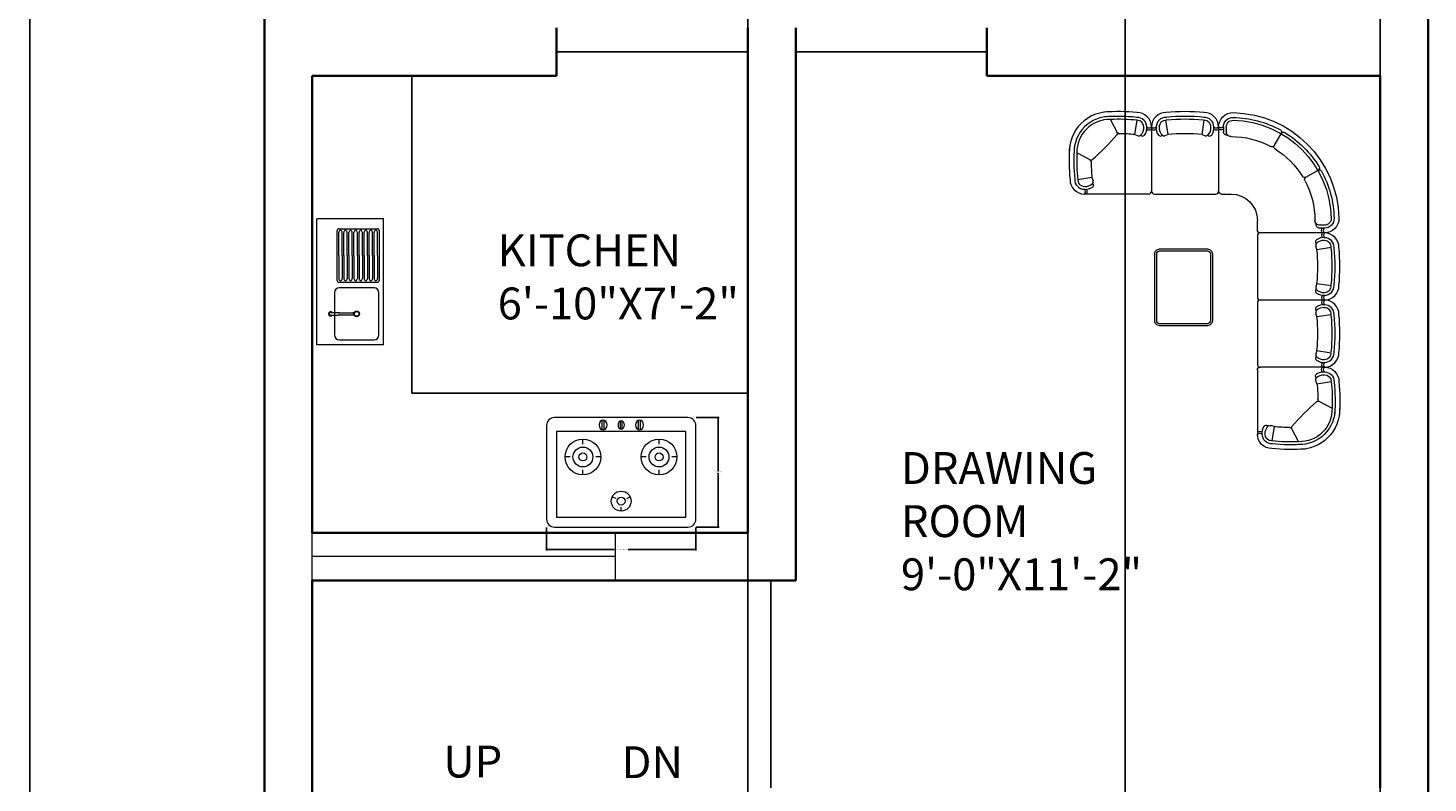
# Model space of a CAD drawing. Units: inches. Extents: x -16 to 587, y -783 to 64.
# Tile 9 of 14: x 279 to 543, y -534 to -392. Entities that reach past the tile are written whole.
import ezdxf

# ---------------------------------------------------------------- set-up
doc = ezdxf.new("R2010")
doc.units = ezdxf.units.IN
doc.header["$MEASUREMENT"] = 0
for name, color, linetype, lineweight in [('A-ANNO-DIMS', 2, 'Continuous', 18), ('A-ANNO-SYMB', 7, 'Continuous', 18), ('A-ANNO-TEXT', 7, 'Continuous', 25), ('A-AREA-IDEN', 7, 'Continuous', 18), ('A-DOOR', 3, 'Continuous', 25), ('A-EQPM', 8, 'Continuous', 18), ('A-FLOR-CASE', 7, 'Continuous', 25), ('A-FLOR-FIXT', 9, 'Continuous', 18), ('A-FURN', 8, 'Continuous', 18), ('A-GLAZ', 4, 'Continuous', 18), ('A-WALL', 7, 'Continuous', 35)]:
    doc.layers.add(name, color=color, linetype=linetype, lineweight=lineweight)
doc.styles.get("Standard").update_dxf_attribs({"font": 'arial.ttf'})
doc.dimstyles.get("Standard").update_dxf_attribs({"dimtxt": 0.18, "dimasz": 0.18, "dimexe": 0.18, "dimexo": 0.0625, "dimgap": 0.09, "dimtad": 0, "dimtih": 1, "dimtoh": 1, "dimdec": 0, "dimzin": 0, "dimdsep": 46, "dimlunit": 3, "dimtxsty": 'Standard', "dimcen": 0.09, "dimadec": 0, "dimazin": 0, "dimtfac": 1, "dimtdec": 0, "dimtofl": 0, "dimtmove": 0, "dimatfit": 3, "dimfxl": 1, "dimtolj": 1, "dimtzin": 0, "dimarcsym": 0})

# ---------------------------------------------------------------- blocks, each defined once
blk = doc.blocks.new('A$C707258B2')
at = {"color": 0}
for p, q in [((0.404, 0.342), (1.074, 0.342)), ((1.104, 0.312), (1.104, 0.212)), ((0.404, 0.292), (0.454, 0.292)), ((0.404, 0.262), (0.454, 0.262)), ((1.479, -0.063), (1.379, -0.063)), ((1.509, -0.763), (1.509, -0.093)), ((0.6, -0.238), (0.47, -0.313)), ((0.929, -0.567), (0.854, -0.697)), ((1.429, -0.763), (1.429, -0.713)), ((1.459, -0.763), (1.459, -0.712))]:
    blk.add_line(p, q, dxfattribs=at)
for centre, radius, start, end in [((0.404, 0.192), 0.15, 90, 181.1754), ((0.378, 0.317), 0.0362, 316.3972, 43.6028), ((0.368, 0.317), 0.0662, 337.8298, 22.1702), ((1.074, 0.312), 0.03, 360, 90), ((1.379, 0.212), 1.125, 181.1754, 268.8246), ((0.404, 0.192), 0.1, 90, 181.1754), ((1.379, 0.212), 1.075, 181.1754, 208.6357), ((0.404, 0.192), 0.07, 90, 181.1754), ((1.379, 0.212), 1.045, 181.1754, 268.8246), ((0.455, 0.256), 0.0357, 345.4262, 90.5555), ((0.454, 0.212), 0.05, 360, 90), ((1.379, 0.212), 0.875, 180, 208.4082), ((1.379, 0.212), 0.275, 180, 270), ((1.479, -0.093), 0.03, 360, 90), ((0.587, -0.216), 0.025, 300, 28.4082), ((0.612, -0.259), 0.025, 31.5918, 120), ((1.379, 0.212), 0.875, 211.5918, 238.4082), ((0.457, -0.291), 0.025, 208.6357, 300), ((0.482, -0.334), 0.025, 120, 211.3643), ((1.379, 0.212), 1.075, 211.3643, 238.6357), ((0.907, -0.555), 0.025, 330, 58.4082), ((0.951, -0.58), 0.025, 61.5918, 150), ((1.379, 0.212), 0.875, 241.5918, 270), ((0.832, -0.685), 0.025, 238.6357, 330), ((0.876, -0.71), 0.025, 150, 241.3643), ((1.379, -0.713), 0.05, 360, 90), ((1.425, -0.709), 0.0336, 354.6301, 109.3883), ((1.379, 0.212), 1.075, 241.3643, 268.8246), ((1.359, -0.763), 0.15, 268.8246, 360), ((1.359, -0.763), 0.1, 268.8246, 360), ((1.359, -0.763), 0.07, 268.8246, 360), ((1.484, -0.799), 0.0662, 67.8298, 112.1702), ((1.484, -0.789), 0.0362, 46.3972, 133.6028)]:
    blk.add_arc(centre, radius, start, end, dxfattribs=at)
blk = doc.blocks.new('A$C1352')
at = {"color": 0}
for points in [[(0.003, 0.053), (0.003, 0.553, -0.414214), (0.053, 0.603), (0.753, 0.603, -0.414214), (0.803, 0.553), (0.803, 0.053, -0.414214), (0.753, 0.003), (0.053, 0.003, -0.414214)], [(0.023, 0.053), (0.023, 0.553, -0.414214), (0.053, 0.583), (0.753, 0.583, -0.414214), (0.783, 0.553), (0.783, 0.053, -0.414214), (0.753, 0.023), (0.053, 0.023, -0.414214)]]:
    blk.add_lwpolyline(points, format="xyb", close=True, dxfattribs=at)
blk = doc.blocks.new('part 01')
at = {"color": 0}
for p, q in [((-670, 700), (0, 700)), ((30, 30), (30, 670)), ((-591, 527), (-740, 550)), ((-591, 527), (-579, 561)), ((-591, 173), (-740, 150)), ((-591, 173), (-579, 139)), ((-670, 0), (0, 0))]:
    blk.add_line(p, q, dxfattribs=at)
for centre, radius, start, end in [((-670, 550), 150, 90, 181.1754), ((-670, 550), 100, 90, 181.1754), ((-670, 550), 70, 90, 181.1754), ((-660, 518), 133, 56.0897, 95.6132), ((-696, 675), 36.2, 316.3972, 43.6028), ((-660, 518), 103, 42.0066, 95.6132), ((-706, 675), 66.2, 337.8298, 22.1702), ((-600, 607), 25, 332.9608, 56.0897), ((-625, 620), 53.2, 321.0017, 332.9608), ((-602, 570), 25, 340, 42.0066), ((0, 670), 30, 0, 90), ((1178, 350), 2008, 174.2835, 185.7165), ((1178, 350), 1958, 174.2835, 185.7165), ((1178, 350), 1928, 174.2835, 185.7165), ((1178, 350), 1778, 174.2835, 185.7165), ((-670, 150), 150, 178.8246, 270), ((-670, 150), 100, 178.8246, 270), ((-670, 150), 70, 178.8246, 270), ((-660, 182), 133, 264.3868, 303.9103), ((-660, 182), 103, 264.3868, 317.9934), ((-696, 25), 36.2, 316.3972, 43.6028), ((-706, 25), 66.2, 337.8298, 22.1702), ((-600, 93), 25, 303.9103, 27.0392), ((-602, 130), 25, 317.9934, 20), ((-625, 80), 53.2, 27.0392, 38.9983), ((0, 30), 30, 270, 0)]:
    blk.add_arc(centre, radius, start, end, dxfattribs=at)
blk = doc.blocks.new('part02')
at = {"color": 0}
for p, q in [((0, -670), (0, 0)), ((30, 30), (700, 30)), ((621, -143), (609, -109)), ((621, -143), (770, -120)), ((640, -326), (778, -399)), ((173, -591), (139, -579)), ((173, -591), (150, -740)), ((356, -610), (429, -748))]:
    blk.add_line(p, q, dxfattribs=at)
for centre, radius, start, end in [((30, 0), 30, 90, 180), ((726, 5), 56.2, 153.6122, 206.6666), ((726, 5), 36.2, 136.3972, 223.6028), ((700, -120), 150, 0, 90), ((630, -63), 25, 123.9103, 207.0392), ((655, -50), 53.2, 207.0392, 218.9983), ((632, -100), 25, 137.9934, 200), ((690, -152), 103, 84.3868, 137.9934), ((689, -151), 132, 85.4378, 123.9887), ((-1148, -320), 1778, 0.3836, 5.7165), ((700, -121), 101, 357.5006, 89.858), ((700, -120), 70, 0, 90), ((-1228, -320), 2008, 357.7349, 5.7032), ((-1148, -320), 1958, 355.8657, 5.7165), ((-1148, -320), 2008, 355.818, 5.7165), ((2220, -2190), 2454, 130.6961, 139.3039), ((439, -409), 419, 268.2181, 1.7819), ((439, -409), 369, 268.2181, 1.7819), ((439, -409), 339, 268.2181, 1.7819), ((632, -344), 20, 62, 130.6961), ((650, -308), 20, 180.3836, 242), ((93, -600), 25, 62.9608, 146.0897), ((182, -660), 103, 132.0066, 185.6132), ((80, -625), 53.2, 51.0017, 62.9608), ((130, -602), 25, 70, 132.0066), ((25, -696), 56.2, 63.3334, 116.3878), ((25, -696), 36.2, 46.3972, 133.6028), ((150, -670), 150, 180, 271.1754), ((182, -660), 133, 146.0897, 185.6132), ((150, -670), 100, 180, 271.1754), ((150, -670), 70, 180, 270), ((350, 1178), 1778, 264.2835, 269.6164), ((338, -620), 20, 28, 89.6164), ((374, -602), 20, 139.3039, 208), ((350, 1258), 2008, 264.2968, 272.2651), ((350, 1178), 2008, 264.2835, 274.182), ((350, 1178), 1958, 264.2835, 274.1343)]:
    blk.add_arc(centre, radius, start, end, dxfattribs=at)
blk = doc.blocks.new('KITCHEN-SINK')
for p, q in [((12.53, 23.71), (0, 23.71)), ((0, 0), (0, 23.71)), ((3.76, 21.39), (3.76, 12.19)), ((4.1, 16.79), (4.1, 21.13)), ((4.19, 21.83), (11.32, 21.83)), ((4.75, 16.79), (4.75, 21.13)), ((5.05, 16.79), (5.05, 21.13)), ((5.7, 16.79), (5.7, 21.13)), ((6, 16.79), (6, 21.13)), ((6.65, 16.79), (6.65, 21.13)), ((6.96, 16.79), (6.96, 21.13)), ((7.6, 16.79), (7.6, 21.13)), ((7.91, 16.79), (7.91, 21.13)), ((8.56, 16.79), (8.56, 21.13)), ((8.86, 16.79), (8.86, 21.13)), ((9.51, 16.79), (9.51, 21.13)), ((9.81, 16.79), (9.81, 21.13)), ((10.46, 16.79), (10.46, 21.13)), ((10.76, 16.79), (10.76, 21.13)), ((11.41, 16.79), (11.41, 21.13)), ((11.75, 12.19), (11.75, 21.39)), ((12.53, 0), (12.53, 23.71)), ((4.1, 16.79), (4.1, 12.45)), ((4.75, 16.79), (4.75, 12.45)), ((5.05, 16.79), (5.05, 12.45)), ((5.7, 16.79), (5.7, 12.45)), ((6, 16.79), (6, 12.45)), ((6.65, 16.79), (6.65, 12.45)), ((6.96, 16.79), (6.96, 12.45)), ((7.6, 16.79), (7.6, 12.45)), ((7.91, 16.79), (7.91, 12.45)), ((8.56, 16.79), (8.56, 12.45)), ((8.86, 16.79), (8.86, 12.45)), ((9.51, 16.79), (9.51, 12.45)), ((9.81, 16.79), (9.81, 12.45)), ((10.46, 16.79), (10.46, 12.45)), ((10.76, 16.79), (10.76, 12.45)), ((11.41, 16.79), (11.41, 12.45)), ((4.19, 11.76), (11.32, 11.76)), ((10.73, 10.7), (4.21, 10.7)), ((3.28, 9.77), (3.28, 6.06)), ((11.66, 1.84), (11.66, 9.77)), ((3.28, 5.95), (3.28, 1.84)), ((4.21, 0.91), (10.73, 0.91)), ((12.53, 0), (0, 0))]:
    blk.add_line(p, q)
for points in [[(2.55, 6.06), (3.98, 6.06)], [(2.55, 5.54), (3.98, 5.54)], [(4.14, 6), (6.76, 6)], [(4.14, 5.61), (6.76, 5.61)]]:
    blk.add_lwpolyline(points)
for radius in [0.54, 0.432]:
    blk.add_circle((7.47, 5.8), radius)
for centre, radius, start, end in [((4.19, 21.39), 0.432, 90, 180), ((4.53, 21.13), 0.432, 104.4903, 180), ((4.32, 21.13), 0.432, 0, 75.5097), ((5.48, 21.13), 0.432, 104.4903, 180), ((5.27, 21.13), 0.432, 0, 75.5097), ((6.44, 21.13), 0.432, 104.4903, 180), ((6.22, 21.13), 0.432, 0, 75.5097), ((7.39, 21.13), 0.432, 104.4903, 180), ((7.17, 21.13), 0.432, 0, 75.5097), ((8.34, 21.13), 0.432, 104.4903, 180), ((8.12, 21.13), 0.432, 0, 75.5097), ((9.29, 21.13), 0.432, 104.4903, 180), ((9.07, 21.13), 0.432, 0, 75.5097), ((10.24, 21.13), 0.432, 104.4903, 180), ((10.03, 21.13), 0.432, 0, 75.5097), ((11.19, 21.13), 0.432, 104.4903, 180), ((10.98, 21.13), 0.432, 0, 75.5097), ((11.32, 21.39), 0.432, 0, 90), ((4.21, 9.77), 0.933, 90, 180), ((4.19, 12.19), 0.432, 180, 270), ((4.53, 12.45), 0.432, 180, 255.5097), ((4.32, 12.45), 0.432, 284.4903, 0), ((5.48, 12.45), 0.432, 180, 255.5097), ((5.27, 12.45), 0.432, 284.4903, 0), ((6.44, 12.45), 0.432, 180, 255.5097), ((6.22, 12.45), 0.432, 284.4903, 0), ((7.39, 12.45), 0.432, 180, 255.5097), ((7.17, 12.45), 0.432, 284.4903, 0), ((8.34, 12.45), 0.432, 180, 255.5097), ((8.12, 12.45), 0.432, 284.4903, 0), ((9.29, 12.45), 0.432, 180, 255.5097), ((9.07, 12.45), 0.432, 284.4903, 0), ((10.24, 12.45), 0.432, 180, 255.5097), ((10.03, 12.45), 0.432, 284.4903, 0), ((10.73, 9.77), 0.933, 0, 90), ((11.19, 12.45), 0.432, 180, 255.5097), ((10.98, 12.45), 0.432, 284.4903, 0), ((11.32, 12.19), 0.432, 270, 0), ((2.55, 5.8), 0.388, 41.9018, 318.0982), ((2.55, 5.8), 0.259, 90, 270), ((3.97, 5.8), 0.259, 272.2198, 87.7802), ((6.78, 5.8), 0.195, 264.9463, 95.0537), ((4.21, 1.84), 0.933, 180, 270), ((10.73, 1.84), 0.933, 270, 0)]:
    blk.add_arc(centre, radius, start, end)
blk = doc.blocks.new('COOKTOP-THREE-BURNER')
for p, q in [((0, 19.11), (0, 1.5)), ((26.61, 20.61), (1.5, 20.61)), ((10.46, 18.28), (10.46, 20.15)), ((10.83, 18.28), (10.83, 20.15)), ((13.92, 18.45), (13.92, 19.97)), ((14.22, 18.45), (14.22, 19.97)), ((17.32, 18.28), (17.32, 20.15)), ((17.7, 18.28), (17.7, 20.15)), ((28.11, 1.5), (28.11, 19.11)), ((26.23, 17.99), (1.87, 17.99)), ((1.87, 17.99), (1.87, 1.87)), ((6.85, 15.63), (6.85, 16.56)), ((21.18, 15.63), (21.18, 16.56)), ((26.23, 1.87), (26.23, 17.99)), ((4.42, 13.19), (3.48, 13.19)), ((10.23, 13.19), (9.29, 13.19)), ((18.74, 13.19), (17.8, 13.19)), ((24.55, 13.19), (23.61, 13.19)), ((6.85, 9.82), (6.85, 10.76)), ((21.18, 9.82), (21.18, 10.76)), ((12.37, 5.69), (13.06, 5.41)), ((15.74, 5.69), (15.08, 5.34)), ((14.05, 3), (14.05, 3.75)), ((1.5, 0), (26.61, 0)), ((1.87, 1.87), (26.23, 1.87))]:
    blk.add_line(p, q)
for centre, radius in [((6.85, 13.19), 3.37), ((21.18, 13.19), 3.37), ((6.85, 13.19), 1.87), ((6.85, 13.19), 0.75), ((21.18, 13.19), 1.87), ((21.18, 13.19), 0.75), ((14.05, 4.88), 1.87), ((14.05, 4.88), 0.75)]:
    blk.add_circle(centre, radius)
for centre, start, end in [((1.5, 19.11), 90, 180), ((26.61, 19.11), 0, 90), ((1.5, 1.5), 180, 270), ((26.61, 1.5), 270, 0)]:
    blk.add_arc(centre, 1.5, start, end)
at = {"extrusion": (0, 0, -1)}
for centre, major_axis in [((10.65, 19.21), (0, 0.937)), ((14.07, 19.21), (0, 0.759)), ((17.51, 19.21), (0, 0.937))]:
    blk.add_ellipse(centre, major_axis=major_axis, ratio=0.802399, dxfattribs=at)
blk = doc.blocks.new('*D40')
at = {"layer": 'A-ANNO-DIMS', "color": 0, "lineweight": -2, "transparency": 16777216}
for p, q in [((376.89, -485.54), (376.89, -489.87)), ((405, -485.54), (405, -489.87)), ((377.07, -489.69), (389.64, -489.69)), ((404.82, -489.69), (392.24, -489.69))]:
    blk.add_line(p, q, dxfattribs=at)
at = {"layer": 'A-ANNO-DIMS', "color": 0, "transparency": 16777216}
for points in [[(377.07, -489.66), (377.07, -489.72), (376.89, -489.69)], [(404.82, -489.66), (404.82, -489.72), (405, -489.69)]]:
    blk.add_solid(points, dxfattribs=at)
at = {"layer": 'Defpoints', "color": 0, "transparency": 16777216}
for p in [(376.89, -485.48), (405, -485.48), (405, -489.69)]:
    blk.add_point(p, dxfattribs=at)
at = {"layer": 'A-ANNO-DIMS', "color": 0, "transparency": 16777216, "insert": (390.94, -489.69), "char_height": 0.18, "attachment_point": 5}
blk.add_mtext('\\A1;COOKTOP 2\'-4" TYP.', dxfattribs=at)
blk = doc.blocks.new('*D41')
at = {"layer": 'A-ANNO-DIMS', "color": 0, "lineweight": -2, "transparency": 16777216}
for p, q in [((405.06, -464.86), (409.39, -464.86)), ((409.21, -465.04), (409.21, -474.99)), ((409.21, -485.3), (409.21, -475.35)), ((405.06, -485.48), (409.39, -485.48))]:
    blk.add_line(p, q, dxfattribs=at)
at = {"layer": 'A-ANNO-DIMS', "color": 0, "transparency": 16777216}
for points in [[(409.18, -465.04), (409.24, -465.04), (409.21, -464.86)], [(409.18, -485.3), (409.24, -485.3), (409.21, -485.48)]]:
    blk.add_solid(points, dxfattribs=at)
at = {"layer": 'Defpoints', "color": 0, "transparency": 16777216}
for p in [(405, -464.86), (409.21, -464.86), (405, -485.48)]:
    blk.add_point(p, dxfattribs=at)
at = {"layer": 'A-ANNO-DIMS', "color": 0, "transparency": 16777216, "insert": (409.21, -475.17), "char_height": 0.18, "attachment_point": 5}
blk.add_mtext('\\A1;1\'-8 1/2" TYP.', dxfattribs=at)
blk = doc.blocks.new('*D53')
at = {"layer": 'A-ANNO-DIMS', "color": 0, "lineweight": -2, "transparency": 16777216}
for p, q in [((323.73, 19.45), (279.46, 19.45)), ((279.64, 19.27), (279.64, -358.87)), ((279.64, -737.37), (279.64, -359.24)), ((323.73, -737.55), (279.46, -737.55))]:
    blk.add_line(p, q, dxfattribs=at)
at = {"layer": 'A-ANNO-DIMS', "color": 0, "transparency": 16777216}
for points in [[(279.61, 19.27), (279.67, 19.27), (279.64, 19.45)], [(279.61, -737.37), (279.67, -737.37), (279.64, -737.55)]]:
    blk.add_solid(points, dxfattribs=at)
at = {"layer": 'Defpoints', "color": 0, "transparency": 16777216}
for p in [(323.79, 19.45), (279.64, -737.55), (323.79, -737.55)]:
    blk.add_point(p, dxfattribs=at)
at = {"layer": 'A-ANNO-DIMS', "color": 0, "transparency": 16777216, "insert": (279.64, -359.05), "char_height": 0.18, "attachment_point": 5}
blk.add_mtext('\\A1;63\'-1"', dxfattribs=at)
blk = doc.blocks.new('*D55')
at = {"layer": 'A-ANNO-DIMS', "color": 0, "lineweight": -2, "transparency": 16777216}
for p, q in [((485.79, -75.62), (485.79, -781.88)), ((533.79, -75.62), (533.79, -781.88)), ((485.97, -781.7), (509.46, -781.7)), ((533.61, -781.7), (510.12, -781.7))]:
    blk.add_line(p, q, dxfattribs=at)
at = {"layer": 'A-ANNO-DIMS', "color": 0, "transparency": 16777216}
for points in [[(485.97, -781.67), (485.97, -781.73), (485.79, -781.7)], [(533.61, -781.67), (533.61, -781.73), (533.79, -781.7)]]:
    blk.add_solid(points, dxfattribs=at)
at = {"layer": 'Defpoints', "color": 0, "transparency": 16777216}
for p in [(485.79, -75.55), (533.79, -75.55), (533.79, -781.7)]:
    blk.add_point(p, dxfattribs=at)
at = {"layer": 'A-ANNO-DIMS', "color": 0, "transparency": 16777216, "insert": (509.79, -781.7), "char_height": 0.18, "attachment_point": 5}
blk.add_mtext('\\A1;4\'-0"', dxfattribs=at)
blk = doc.blocks.new('*D59')
at = {"layer": 'A-ANNO-DIMS', "color": 0, "lineweight": -2, "transparency": 16777216}
for p, q in [((414.79, -712.99), (414.79, 63.78)), ((414.97, 63.6), (478.4, 63.6)), ((542.61, 63.6), (479.18, 63.6)), ((542.79, -712.99), (542.79, 63.78))]:
    blk.add_line(p, q, dxfattribs=at)
at = {"layer": 'A-ANNO-DIMS', "color": 0, "transparency": 16777216}
for points in [[(414.97, 63.63), (414.97, 63.57), (414.79, 63.6)], [(542.61, 63.63), (542.61, 63.57), (542.79, 63.6)]]:
    blk.add_solid(points, dxfattribs=at)
at = {"layer": 'Defpoints', "color": 0, "transparency": 16777216}
for p in [(542.79, 63.6), (414.79, -713.05), (542.79, -713.05)]:
    blk.add_point(p, dxfattribs=at)
at = {"layer": 'A-ANNO-DIMS', "color": 0, "transparency": 16777216, "insert": (478.79, 63.6), "char_height": 0.18, "attachment_point": 5}
blk.add_mtext('\\A1;10\'-8"', dxfattribs=at)

msp = doc.modelspace()

# ---------------------------------------------------------------- linework, layer by layer
at = {"layer": 'A-ANNO-SYMB'}
msp.add_line((359.58, -529.79), (359.58, -529.79), dxfattribs=at)
at = {"layer": 'A-DOOR'}
for p, q in [((378.79, -396.05), (414.79, -396.05)), ((423.79, -396.05), (459.79, -396.05)), ((419.12, -534.55), (419.12, -495.55))]:
    msp.add_line(p, q, dxfattribs=at)
at = {"layer": 'A-FLOR-CASE'}
for p, q in [((351.52, -400.55), (351.52, -460.28)), ((351.52, -460.28), (414.79, -460.28))]:
    msp.add_line(p, q, dxfattribs=at)
at = {"layer": 'A-GLAZ'}
for p, q in [((332.79, -495.55), (332.79, -486.55)), ((332.79, -486.55), (389.81, -486.55)), ((389.81, -486.55), (389.81, -495.55)), ((389.81, -491.05), (332.79, -491.05)), ((389.81, -495.55), (332.79, -495.55))]:
    msp.add_line(p, q, dxfattribs=at)
at = {"layer": 'A-WALL'}
for p, q in [((323.79, 19.45), (323.79, -737.55)), ((542.79, 19.45), (542.79, -737.55)), ((378.79, -391.55), (378.79, -400.55)), ((414.79, -391.55), (414.79, -486.55)), ((423.79, -391.55), (423.79, -495.55)), ((459.79, -391.55), (459.79, -400.55)), ((332.79, -400.55), (378.79, -400.55)), ((332.79, -400.55), (332.79, -486.55)), ((459.79, -400.55), (476.79, -400.55)), ((476.79, -400.55), (533.79, -400.55)), ((533.79, -400.55), (533.79, -486.55)), ((332.79, -486.55), (414.79, -486.55)), ((533.79, -486.55), (533.79, -495.55)), ((332.79, -495.55), (423.79, -495.55)), ((332.79, -495.55), (332.79, -663.55)), ((533.79, -495.55), (533.79, -534.55))]:
    msp.add_line(p, q, dxfattribs=at)

# ---------------------------------------------------------------- block references
at = {"layer": 'A-EQPM'}
msp.add_blockref('COOKTOP-THREE-BURNER', (376.89, -485.48), dxfattribs=at)
at = {"layer": 'A-FLOR-FIXT'}
msp.add_blockref('KITCHEN-SINK', (333.69, -451.16), dxfattribs=at)
at = {"layer": 'A-FURN', "ltscale": 0.03}
for name, p, xscale, yscale, zscale, rotation in [('part02', (490.75, -422.27), 0.0180440482994306, 0.0180440482994306, 0.0180440482994306, 180), ('part 01', (490.75, -422.27), 0.0180440482994306, 0.0180440482994306, 0.0180440482994306, 270), ('A$C707258B2', (509.55, -402.89), -18.04404829943058, 18.04404829943058, 18.04404829943058, 89.9999999999967), ('part 01', (511.23, -430.12), 0.0180440482994306, 0.0180440482994306, 0.0180440482994306, 180), ('A$C1352', (491.32, -433.09), 18.04404829943058, 18.04404829943058, 18.04404829943058, 270), ('part 01', (511.23, -442.75), 0.0180440482994306, 0.0180440482994306, 0.0180440482994306, 180), ('part02', (511.23, -455.38), -0.0180440482994306, 0.0180440482994306, 0.0180440482994306, 89.9999999999967)]:
    msp.add_blockref(name, p, dxfattribs=dict(at, xscale=xscale, yscale=yscale, zscale=zscale, rotation=rotation))

# ---------------------------------------------------------------- texts
at = {"layer": 'A-ANNO-TEXT', "char_height": 6, "attachment_point": 1}
for s, insert in [('UP', (357.46, -526.61)), ('DN', (391.01, -526.74))]:
    msp.add_mtext(s, dxfattribs=dict(at, insert=insert))
at = {"layer": 'A-AREA-IDEN', "char_height": 6, "attachment_point": 1}
for s, insert in [('KITCHEN\\P6\'-10"X7\'-2"', (367.7, -430.4)), ('DRAWING\\PROOM\\P9\'-0"X11\'-2"', (443.59, -471.37))]:
    msp.add_mtext(s, dxfattribs=dict(at, insert=insert))

# ---------------------------------------------------------------- dimensions: what is measured, and where the dimension line sits
at = {"layer": 'A-ANNO-DIMS'}
for base, p1, p2, picture, middle in [((542.79, 63.6), (414.79, -713.05), (542.79, -713.05), '*D59', (478.79, 63.6)), ((533.79, -781.7), (485.79, -75.55), (533.79, -75.55), '*D55', (509.79, -781.7))]:
    dim = msp.add_linear_dim(base=base, p1=p1, p2=p2, dimstyle='Standard', override={"dimdec": 1, "dimlfac": 1, "dimrnd": 0, "dimzin": 1, "dimdsep": 46, "dimlunit": 4, "dimfrac": 2}, dxfattribs=at)
    dim.commit()
    dim.dimension.update_dxf_attribs({"geometry": picture, "text_midpoint": middle})
dim = msp.add_linear_dim(base=(279.64, -737.55), p1=(323.79, 19.45), p2=(323.79, -737.55), angle=90, dimstyle='Standard', override={"dimdec": 1, "dimlfac": 1, "dimrnd": 0, "dimzin": 1, "dimdsep": 46, "dimlunit": 4, "dimfrac": 2}, dxfattribs=at)
dim.commit()
dim.dimension.update_dxf_attribs({"geometry": '*D53', "text_midpoint": (279.64, -359.05)})
dim = msp.add_linear_dim(base=(409.21, -464.86), p1=(405, -485.48), p2=(405, -464.86), angle=90, text='<> TYP.', dimstyle='Standard', override={"dimdec": 1, "dimlfac": 1, "dimrnd": 0, "dimzin": 1, "dimdsep": 46, "dimlunit": 4, "dimfrac": 2}, dxfattribs=at)
dim.commit()
dim.dimension.update_dxf_attribs({"geometry": '*D41', "text_midpoint": (409.21, -475.17)})
dim = msp.add_linear_dim(base=(405, -489.69), p1=(376.89, -485.48), p2=(405, -485.48), text='COOKTOP <> TYP.', dimstyle='Standard', override={"dimdec": 1, "dimlfac": 1, "dimrnd": 0, "dimzin": 1, "dimdsep": 46, "dimlunit": 4, "dimfrac": 2}, dxfattribs=at)
dim.commit()
dim.dimension.update_dxf_attribs({"geometry": '*D40', "text_midpoint": (390.94, -489.69)})

doc.saveas('drawing.dxf')
